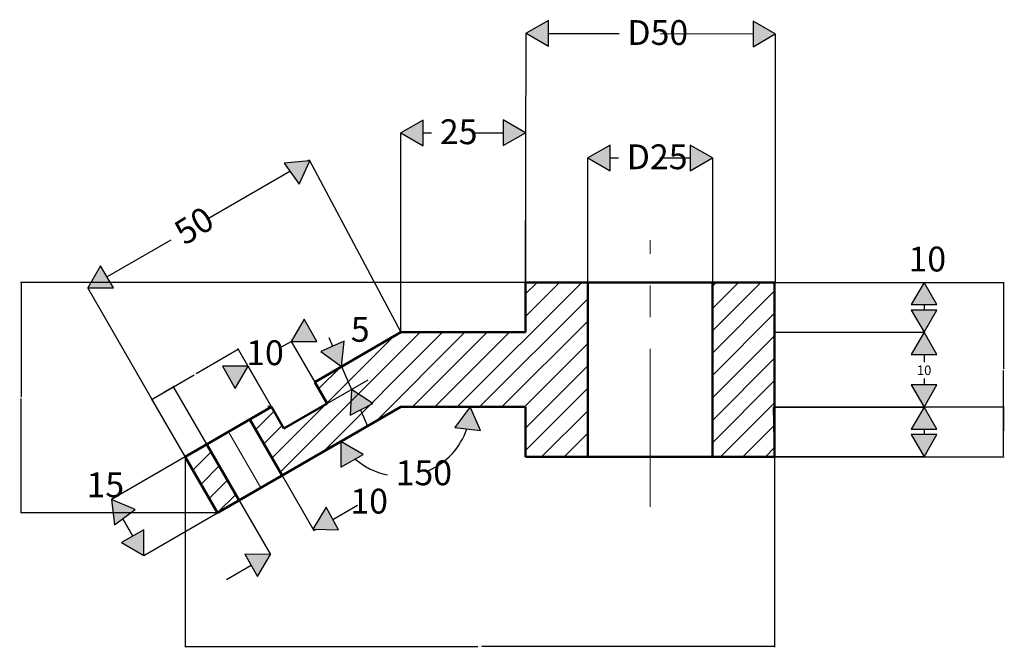
# Model space of a CAD drawing. Units: millimetres. Extents: x 537 to 734, y 1281 to 1407.
import ezdxf

# ---------------------------------------------------------------- set-up
doc = ezdxf.new("R2010")
doc.units = ezdxf.units.MM
doc.linetypes.add('CENTER', pattern=[50.8, 31.75, -6.35, 6.35, -6.35])
for name, color, linetype, lineweight in [('M-CNTR', 4, 'CENTER', 18), ('M-DIMS', 2, 'Continuous', 25), ('M-HATC', 8, 'Continuous', 18), ('M-OUTL', 7, 'Continuous', 50), ('M-TEXT', 7, 'Continuous', 25)]:
    doc.layers.add(name, color=color, linetype=linetype, lineweight=lineweight)
doc.styles.get("Standard").update_dxf_attribs({"font": 'arial.ttf'})
doc.dimstyles.get("Standard").update_dxf_attribs({"dimtxt": 0.18, "dimasz": 0.18, "dimexe": 0.18, "dimexo": 0.0625, "dimgap": 0.09, "dimtad": 0, "dimtih": 1, "dimtoh": 1, "dimdec": 4, "dimzin": 0, "dimdsep": 46, "dimtxsty": 'Standard', "dimcen": 0.09, "dimadec": 0, "dimazin": 0, "dimtfac": 1, "dimtdec": 4, "dimtofl": 0, "dimtmove": 0, "dimatfit": 3, "dimfxl": 1, "dimtolj": 1, "dimtzin": 0, "dimarcsym": 0})

# ---------------------------------------------------------------- blocks, each defined once
blk = doc.blocks.new('*D1')
at = {"layer": 'Defpoints', "color": 0, "transparency": 16777216}
for p in [(569.87, 1319.42), (688.17, 1319.42), (688.17, 1281.37)]:
    blk.add_point(p, dxfattribs=at)
at = {"layer": 'M-DIMS', "color": 0, "lineweight": -2, "transparency": 16777216}
for p, q in [((569.87, 1319.35), (569.87, 1281.19)), ((688.17, 1319.35), (688.17, 1281.19)), ((570.05, 1281.37), (628.63, 1281.37)), ((687.99, 1281.37), (629.4, 1281.37))]:
    blk.add_line(p, q, dxfattribs=at)
at = {"layer": 'M-DIMS', "color": 0, "transparency": 16777216}
for points in [[(570.05, 1281.4), (570.05, 1281.34), (569.87, 1281.37)], [(687.99, 1281.4), (687.99, 1281.34), (688.17, 1281.37)]]:
    blk.add_solid(points, dxfattribs=at)
at = {"layer": 'M-DIMS', "color": 0, "transparency": 16777216, "insert": (629.02, 1281.37), "char_height": 0.18, "attachment_point": 5}
blk.add_mtext('\\A1;118.3', dxfattribs=at)
blk = doc.blocks.new('*D2')
at = {"layer": 'Defpoints', "color": 0, "transparency": 16777216}
for p in [(536.95, 1354.42), (638.17, 1354.42), (576.36, 1308.17)]:
    blk.add_point(p, dxfattribs=at)
at = {"layer": 'M-DIMS', "color": 0, "lineweight": -2, "transparency": 16777216}
for p, q in [((638.11, 1354.42), (536.77, 1354.42)), ((536.95, 1354.24), (536.95, 1331.47)), ((536.95, 1308.35), (536.95, 1331.11)), ((576.3, 1308.17), (536.77, 1308.17))]:
    blk.add_line(p, q, dxfattribs=at)
at = {"layer": 'M-DIMS', "color": 0, "transparency": 16777216}
for points in [[(536.92, 1354.24), (536.98, 1354.24), (536.95, 1354.42)], [(536.92, 1308.35), (536.98, 1308.35), (536.95, 1308.17)]]:
    blk.add_solid(points, dxfattribs=at)
at = {"layer": 'M-DIMS', "color": 0, "transparency": 16777216, "insert": (536.95, 1331.29), "char_height": 0.18, "attachment_point": 5}
blk.add_mtext('\\A1;46.25', dxfattribs=at)
blk = doc.blocks.new('*D3')
at = {"layer": 'Defpoints', "color": 0, "transparency": 16777216}
for p in [(580.51, 1340.98), (587.19, 1329.42), (569.87, 1319.42)]:
    blk.add_point(p, dxfattribs=at)
at = {"layer": 'M-DIMS', "color": 0, "lineweight": -2, "transparency": 16777216}
for p, q in [((580.36, 1340.89), (572.07, 1336.1)), ((587.16, 1329.47), (580.42, 1341.13)), ((563.35, 1331.07), (571.63, 1335.85)), ((569.84, 1319.47), (563.1, 1331.13))]:
    blk.add_line(p, q, dxfattribs=at)
at = {"layer": 'M-DIMS', "color": 0, "transparency": 16777216}
for points in [[(580.34, 1340.91), (580.37, 1340.86), (580.51, 1340.98)], [(563.33, 1331.09), (563.36, 1331.04), (563.19, 1330.98)]]:
    blk.add_solid(points, dxfattribs=at)
at = {"layer": 'M-DIMS', "color": 0, "transparency": 16777216, "insert": (571.85, 1335.98), "char_height": 0.18, "attachment_point": 5}
blk.add_mtext('\\A1;20', dxfattribs=at)
blk = doc.blocks.new('*D4')
at = {"layer": 'Defpoints', "color": 0, "transparency": 16777216}
for p in [(567.52, 1333.48), (574.2, 1321.92), (569.87, 1319.42)]:
    blk.add_point(p, dxfattribs=at)
at = {"layer": 'M-DIMS', "color": 0, "lineweight": -2, "transparency": 16777216}
for p, q in [((563.35, 1331.07), (565.21, 1332.14)), ((567.37, 1333.39), (565.51, 1332.31)), ((574.17, 1321.97), (567.43, 1333.63)), ((569.84, 1319.47), (563.1, 1331.13))]:
    blk.add_line(p, q, dxfattribs=at)
at = {"layer": 'M-DIMS', "color": 0, "transparency": 16777216}
for points in [[(567.35, 1333.41), (567.38, 1333.36), (567.52, 1333.48)], [(563.33, 1331.09), (563.36, 1331.04), (563.19, 1330.98)]]:
    blk.add_solid(points, dxfattribs=at)
at = {"layer": 'M-DIMS', "color": 0, "transparency": 16777216, "insert": (565.36, 1332.23), "char_height": 0.18, "attachment_point": 5}
blk.add_mtext('\\A1;5', dxfattribs=at)
blk = doc.blocks.new('*D5')
at = {"layer": 'Defpoints', "color": 0, "transparency": 16777216}
for p in [(688.17, 1329.42), (734.1, 1329.42), (688.17, 1319.42)]:
    blk.add_point(p, dxfattribs=at)
at = {"layer": 'M-DIMS', "color": 0, "lineweight": -2, "transparency": 16777216}
for p, q in [((688.23, 1329.42), (734.28, 1329.42)), ((734.1, 1329.24), (734.1, 1324.6)), ((734.1, 1319.6), (734.1, 1324.23)), ((688.23, 1319.42), (734.28, 1319.42))]:
    blk.add_line(p, q, dxfattribs=at)
at = {"layer": 'M-DIMS', "color": 0, "transparency": 16777216}
for points in [[(734.07, 1329.24), (734.13, 1329.24), (734.1, 1329.42)], [(734.07, 1319.6), (734.13, 1319.6), (734.1, 1319.42)]]:
    blk.add_solid(points, dxfattribs=at)
at = {"layer": 'M-DIMS', "color": 0, "transparency": 16777216, "insert": (734.1, 1324.42), "char_height": 0.18, "attachment_point": 5}
blk.add_mtext('\\A1;10', dxfattribs=at)
blk = doc.blocks.new('*D6')
at = {"layer": 'Defpoints', "color": 0, "transparency": 16777216}
for p in [(688.17, 1354.42), (734.1, 1354.42), (688.17, 1319.42)]:
    blk.add_point(p, dxfattribs=at)
at = {"layer": 'M-DIMS', "color": 0, "lineweight": -2, "transparency": 16777216}
for p, q in [((688.23, 1354.42), (734.28, 1354.42)), ((734.1, 1354.24), (734.1, 1337.1)), ((734.1, 1319.6), (734.1, 1336.73)), ((688.23, 1319.42), (734.28, 1319.42))]:
    blk.add_line(p, q, dxfattribs=at)
at = {"layer": 'M-DIMS', "color": 0, "transparency": 16777216}
for points in [[(734.07, 1354.24), (734.13, 1354.24), (734.1, 1354.42)], [(734.07, 1319.6), (734.13, 1319.6), (734.1, 1319.42)]]:
    blk.add_solid(points, dxfattribs=at)
at = {"layer": 'M-DIMS', "color": 0, "transparency": 16777216, "insert": (734.1, 1336.92), "char_height": 0.18, "attachment_point": 5}
blk.add_mtext('\\A1;35', dxfattribs=at)

msp = doc.modelspace()

# ---------------------------------------------------------------- hatches: boundary and pattern name
at = {"layer": 'M-DIMS'}
h = msp.add_hatch(color=256, dxfattribs=at)
h.dxf.hatch_style = 1
h.paths.add_polyline_path([(720.746, 1323.878), (715.594, 1323.878), (718.17, 1319.416)])
h.paths.add_polyline_path([(715.594, 1324.953), (720.746, 1324.953), (718.17, 1329.414)])
h.paths.add_polyline_path([(718.17, 1329.414), (720.746, 1333.876), (715.594, 1333.876)])
h.paths.add_polyline_path([(715.594, 1339.955), (720.746, 1339.955), (718.17, 1344.416)])
h.paths.add_polyline_path([(718.17, 1344.416), (720.746, 1348.878), (715.594, 1348.878)])
h.paths.add_polyline_path([(718.17, 1354.416), (715.594, 1349.955), (720.746, 1349.955)])
h.paths.add_polyline_path([(581.809, 1299.863), (584.341, 1295.376), (586.961, 1299.812)])
h.paths.add_polyline_path([(595.519, 1304.988), (595.569, 1304.902), (600.62, 1304.796), (598.138, 1309.311)])
h.paths.add_polyline_path([(605.587, 1319.886), (601.126, 1322.462), (601.126, 1317.31)])
h.paths.add_polyline_path([(629.116, 1324.685), (627.078, 1329.416), (624, 1325.285)])
h.paths.add_polyline_path([(559.797, 1308.828), (555.067, 1310.871), (555.664, 1305.753)])
h.paths.add_polyline_path([(557.101, 1302.197), (561.562, 1299.621), (561.562, 1304.773)])
h.paths.add_polyline_path([(582.472, 1337.588), (577.32, 1337.588), (579.896, 1333.126)])
h.paths.add_polyline_path([(591.132, 1342.588), (596.284, 1342.588), (593.708, 1347.049)])
h.paths.add_polyline_path([(555.448, 1353.318), (552.872, 1357.78), (550.296, 1353.318)])
h.paths.add_polyline_path([(589.731, 1378.341), (592.726, 1374.15), (594.859, 1378.84)])
h.paths.add_polyline_path([(617.632, 1386.992), (613.17, 1384.416), (617.632, 1381.84)])
h.paths.add_polyline_path([(633.708, 1387.047), (633.708, 1381.895), (638.17, 1384.471)])
h.paths.add_polyline_path([(638.295, 1404.416), (642.757, 1401.84), (642.757, 1406.992)])
h.paths.add_polyline_path([(683.833, 1406.867), (683.833, 1401.715), (688.295, 1404.291)])
h.paths.add_polyline_path([(675.67, 1379.416), (671.208, 1381.992), (671.208, 1376.84)])
h.paths.add_polyline_path([(655.132, 1376.84), (655.132, 1381.992), (650.67, 1379.416)])
h.paths.add_polyline_path([(601.575, 1339.793), (607.934, 1339.793), (607.934, 1350.054), (601.575, 1350.054)], flags=9)
h = msp.add_hatch(color=256, dxfattribs=at)
h.dxf.hatch_style = 1
h.paths.add_polyline_path([(601.79, 1342.637), (597.071, 1340.571), (601.22, 1337.517)])
h.paths.add_polyline_path([(607.548, 1330.086), (603.237, 1332.908), (602.948, 1327.764)])
at = {"layer": 'M-HATC'}
h = msp.add_hatch(dxfattribs=at)
h.set_pattern_fill('ANSI31', color=256)
h.paths.add_polyline_path([(574.199, 1321.916), (569.869, 1319.416), (576.364, 1308.166), (580.694, 1310.666)])
h.paths.add_polyline_path([(613.17, 1329.416), (638.17, 1329.416), (638.17, 1319.416), (650.67, 1319.416), (650.67, 1354.416), (638.17, 1354.416), (638.17, 1344.416), (613.17, 1344.416), (595.85, 1334.416), (598.35, 1330.086), (589.689, 1325.086), (587.189, 1329.416), (582.859, 1326.916), (589.354, 1315.666)])
h.paths.add_polyline_path([(688.17, 1344.416), (688.17, 1354.416), (675.67, 1354.416), (675.67, 1319.416), (688.17, 1319.416), (688.17, 1329.416)])
h.paths.add_polyline_path([(602.948, 1327.764), (607.548, 1330.086), (603.237, 1332.908)], flags=0)

# ---------------------------------------------------------------- linework, layer by layer
at = {"layer": 'M-CNTR'}
for p, q in [((663.17, 1309.36), (663.17, 1362.896)), ((578.529, 1324.416), (585.024, 1313.166)), ((663.17, 1319.416), (663.17, 1309.36))]:
    msp.add_line(p, q, dxfattribs=at)
at = {"layer": 'M-DIMS'}
for p, q in [((638.17, 1354.416), (638.295, 1404.416)), ((642.757, 1404.405), (656.944, 1404.37)), ((665.243, 1404.349), (683.833, 1404.302)), ((688.295, 1404.291), (688.295, 1354.416)), ((613.17, 1344.416), (613.17, 1384.416)), ((617.632, 1384.426), (619.319, 1384.43)), ((627.619, 1384.448), (633.708, 1384.461)), ((638.17, 1384.471), (638.17, 1354.416)), ((594.429, 1378.798), (594.775, 1378.998)), ((594.775, 1378.998), (613.17, 1344.416)), ((650.67, 1354.416), (650.67, 1379.416)), ((655.132, 1379.416), (656.819, 1379.416)), ((665.119, 1379.416), (671.208, 1379.416)), ((675.67, 1379.416), (675.67, 1354.416)), ((574.205, 1367.122), (590.872, 1376.745)), ((554.16, 1355.549), (567.012, 1362.969)), ((688.17, 1354.416), (718.17, 1354.416)), ((569.869, 1319.416), (550.296, 1353.318)), ((718.17, 1349.955), (718.17, 1348.878)), ((688.17, 1344.416), (718.17, 1344.416)), ((588.75, 1341.213), (591.132, 1342.588)), ((591.132, 1342.588), (595.85, 1334.416)), ((598.674, 1343.332), (599.43, 1341.604)), ((718.17, 1339.955), (718.17, 1338.387)), ((587.189, 1329.416), (582.472, 1337.588)), ((601.22, 1337.517), (603.237, 1332.908)), ((598.35, 1330.086), (606.584, 1334.84)), ((718.17, 1335.151), (718.17, 1333.876)), ((605.03, 1328.815), (606.462, 1325.543)), ((688.17, 1319.416), (687.971, 1329.414)), ((687.971, 1329.414), (718.17, 1329.414)), ((718.17, 1324.953), (718.17, 1323.878)), ((569.869, 1319.416), (555.067, 1310.871)), ((718.17, 1319.416), (688.17, 1319.416)), ((589.354, 1315.666), (595.71, 1304.658)), ((580.694, 1310.666), (586.961, 1299.812)), ((599.494, 1306.843), (604.47, 1309.716)), ((557.313, 1306.98), (559.332, 1303.485)), ((559.332, 1303.485), (557.313, 1306.98)), ((557.313, 1306.98), (559.332, 1303.485)), ((561.562, 1299.621), (576.364, 1308.166)), ((595.71, 1304.658), (596.113, 1304.891)), ((583.097, 1297.581), (578.135, 1294.717))]:
    msp.add_line(p, q, dxfattribs=at)
for points in [[(638.295, 1404.416), (642.757, 1401.84), (642.757, 1406.992)], [(688.295, 1404.291), (683.833, 1406.867), (683.833, 1401.715)], [(613.17, 1384.416), (617.632, 1381.84), (617.632, 1386.992)], [(638.17, 1384.471), (633.708, 1387.047), (633.708, 1381.895)], [(650.67, 1379.416), (655.132, 1376.84), (655.132, 1381.992)], [(675.67, 1379.416), (671.208, 1381.992), (671.208, 1376.84)], [(589.731, 1378.341), (592.726, 1374.15), (594.859, 1378.84)], [(550.296, 1353.318), (555.448, 1353.318), (552.872, 1357.78)], [(718.17, 1354.416), (715.594, 1349.955), (720.746, 1349.955)], [(718.17, 1344.416), (720.746, 1348.878), (715.594, 1348.878)], [(591.132, 1342.588), (596.284, 1342.588), (593.708, 1347.049)], [(718.17, 1344.416), (715.594, 1339.955), (720.746, 1339.955)], [(601.22, 1337.517), (601.79, 1342.637), (597.071, 1340.571)], [(582.472, 1337.588), (577.32, 1337.588), (579.896, 1333.126)], [(603.237, 1332.908), (602.948, 1327.764), (607.548, 1330.086)], [(718.17, 1329.414), (720.746, 1333.876), (715.594, 1333.876)], [(629.116, 1324.685), (627.078, 1329.416), (624, 1325.285)], [(718.17, 1329.414), (715.594, 1324.953), (720.746, 1324.953)], [(605.587, 1319.886), (601.126, 1322.462), (601.126, 1317.31)], [(718.17, 1319.416), (720.746, 1323.878), (715.594, 1323.878)], [(555.067, 1310.871), (555.664, 1305.753), (559.797, 1308.828)], [(595.469, 1304.904), (600.62, 1304.796), (598.138, 1309.311)], [(561.562, 1299.621), (561.562, 1304.773), (557.101, 1302.197)], [(586.961, 1299.812), (581.809, 1299.863), (584.341, 1295.376)]]:
    msp.add_lwpolyline(points, close=True, dxfattribs=at)
for start, end in [(293.63363, 341.52068), (228.71197, 258.70513)]:
    msp.add_arc((613.17, 1329.416), 13.908, start, end, dxfattribs=at)
at = {"layer": 'M-OUTL'}
for p, q in [((638.17, 1354.416), (688.17, 1354.416)), ((638.17, 1354.416), (638.17, 1344.416)), ((638.17, 1344.416), (638.17, 1354.416)), ((663.17, 1354.416), (650.67, 1354.416)), ((650.67, 1354.416), (650.67, 1319.416)), ((663.17, 1354.416), (675.67, 1354.416)), ((675.67, 1354.416), (675.67, 1319.416)), ((688.17, 1344.416), (688.17, 1354.416)), ((613.17, 1344.416), (595.85, 1334.416)), ((638.17, 1344.416), (613.17, 1344.416)), ((638.17, 1344.416), (613.17, 1344.416)), ((688.17, 1329.416), (688.17, 1344.416)), ((595.85, 1334.416), (598.35, 1330.086)), ((587.189, 1329.416), (569.869, 1319.416)), ((613.17, 1329.416), (576.364, 1308.166)), ((587.189, 1329.416), (586.476, 1329.416)), ((587.189, 1329.416), (589.689, 1325.086)), ((598.35, 1330.086), (589.689, 1325.086)), ((638.17, 1329.416), (613.17, 1329.416)), ((638.17, 1319.416), (638.17, 1329.416)), ((688.17, 1319.416), (688.17, 1329.416)), ((582.859, 1326.916), (589.354, 1315.666)), ((574.199, 1321.916), (580.694, 1310.666)), ((569.869, 1319.416), (576.364, 1308.166)), ((688.17, 1319.416), (638.17, 1319.416))]:
    msp.add_line(p, q, dxfattribs=at)

# ---------------------------------------------------------------- texts
at = {"layer": 'M-TEXT', "attachment_point": 1}
for s, width, gutter_width, insert, char_height in [('D50', 4.97962, 24.898, (658.604, 1407.059), 4.9796), ('25', 4.97962, 24.898, (620.979, 1387.149), 4.9796), ('D25', 4.97962, 24.898, (658.479, 1382.122), 4.9796), ('10', 4.97962, 24.898, (715.056, 1361.597), 4.9796), ('5', 4.97962, 24.898, (603.109, 1347.491), 4.98), ('10', 4.97962, 24.898, (582.111, 1342.793), 4.9796), ('10', 1.91735, 9.587, (716.728, 1337.748), 1.9173), ('150', 4.97962, 24.898, (612.106, 1318.695), 4.9796), ('15', 4.97962, 24.898, (550.061, 1316.282), 4.9796), ('10', 4.97962, 24.898, (603.016, 1313.007), 4.9796)]:
    msp.add_mtext_dynamic_manual_height_columns(s, width=width, gutter_width=gutter_width, heights=[0], dxfattribs=dict(at, insert=insert, char_height=char_height))
at = {"layer": 'M-TEXT', "insert": (567.105, 1365.939), "char_height": 4.9796, "attachment_point": 1, "rotation": 32.17629}
msp.add_mtext_dynamic_manual_height_columns('50', width=4.97962, gutter_width=24.898, heights=[0], dxfattribs=at)

# ---------------------------------------------------------------- dimensions: what is measured, and where the dimension line sits
at = {"layer": 'M-DIMS'}
for base, p1, p2, angle, override, picture, middle in [((536.946, 1354.416), (576.364, 1308.166), (638.17, 1354.416), 90, {"dimdec": 2, "dimlfac": 1, "dimrnd": 0, "dimzin": 0, "dimdsep": 46, "dimlunit": 2}, '*D2', (536.946, 1331.291)), ((734.096, 1354.416), (688.17, 1319.416), (688.17, 1354.416), 90, {"dimdec": 0, "dimlfac": 1, "dimrnd": 0, "dimzin": 0, "dimdsep": 46, "dimlunit": 2}, '*D6', (734.096, 1336.916)), ((580.514, 1340.978), (569.869, 1319.416), (587.189, 1329.416), 30, {"dimdec": 0, "dimlfac": 1, "dimrnd": 0, "dimzin": 0, "dimdsep": 46, "dimlunit": 2}, '*D3', (571.854, 1335.978)), ((567.524, 1333.478), (569.869, 1319.416), (574.199, 1321.916), 30, {"dimdec": 0, "dimlfac": 1, "dimrnd": 0, "dimzin": 0, "dimdsep": 46, "dimlunit": 2}, '*D4', (565.359, 1332.228)), ((734.096, 1329.416), (688.17, 1319.416), (688.17, 1329.416), 90, {"dimdec": 0, "dimlfac": 1, "dimrnd": 0, "dimzin": 0, "dimdsep": 46, "dimlunit": 2}, '*D5', (734.096, 1324.416))]:
    dim = msp.add_linear_dim(base=base, p1=p1, p2=p2, angle=angle, dimstyle='Standard', override=override, dxfattribs=at)
    dim.commit()
    dim.dimension.update_dxf_attribs({"geometry": picture, "text_midpoint": middle})
dim = msp.add_linear_dim(base=(688.17, 1281.367), p1=(569.869, 1319.416), p2=(688.17, 1319.416), dimstyle='Standard', override={"dimdec": 1, "dimlfac": 1, "dimrnd": 0, "dimzin": 0, "dimdsep": 46, "dimlunit": 2}, dxfattribs=at)
dim.commit()
dim.dimension.update_dxf_attribs({"geometry": '*D1', "text_midpoint": (629.019, 1281.367)})

doc.saveas('drawing.dxf')
